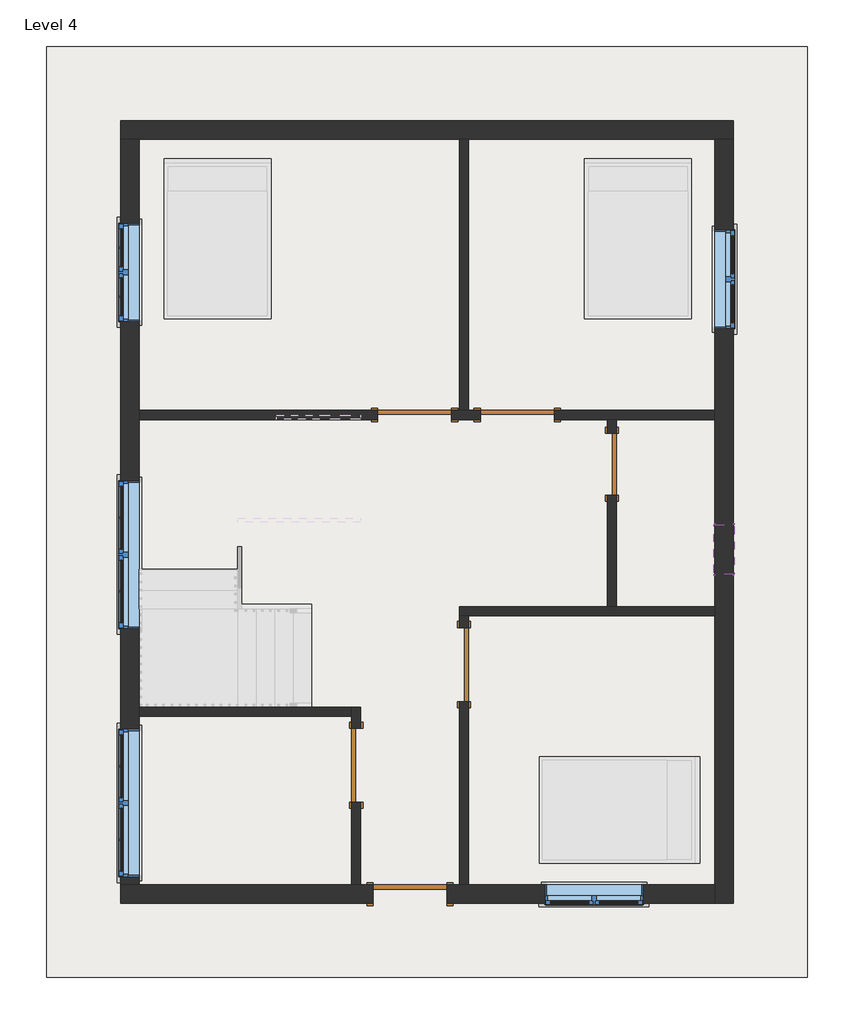
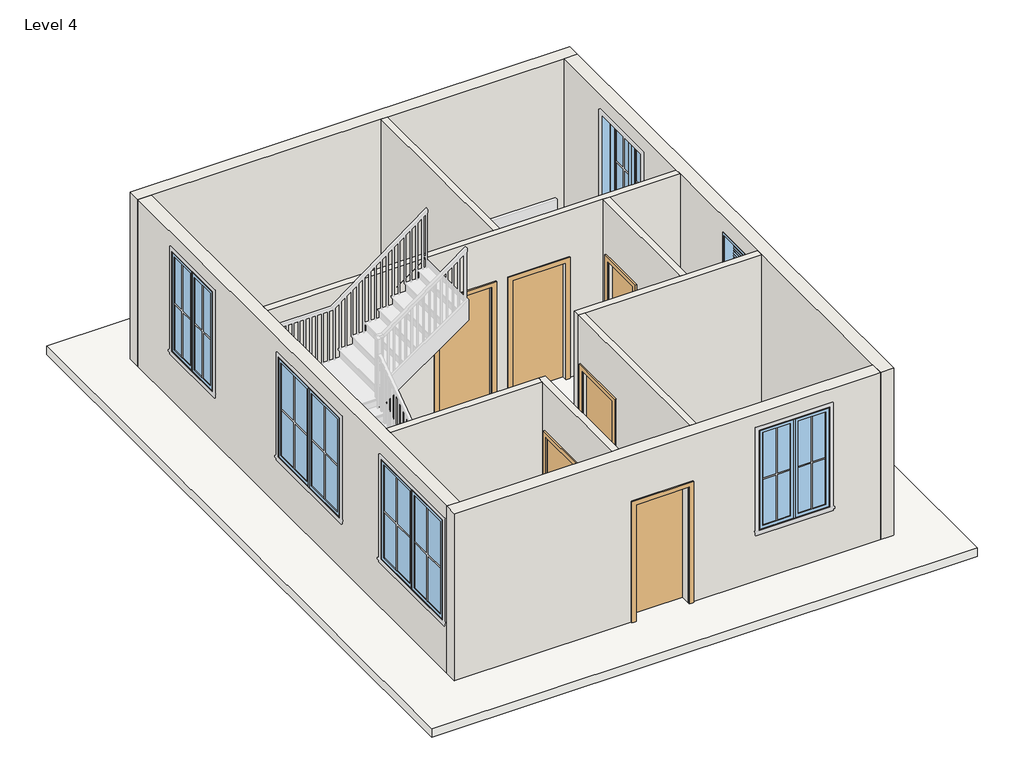
# One storey, part 1 of 3: 11 walls, 6 doors, 6 windows, 1 roof.
"""IFC4 building model written with IfcOpenShell, lengths in millimetres."""

from ifc_helpers import new_model, si_unit, frame, origin, place, context, project, spatial, polyline, outline, extrude, faceted_brep, transform, mapped, element, save
from components import door_f2b275c1, single_flush_door_3_e5f9f3c4, single_flush_door_3_305aa2a5, single_flush_door_3_a90ba1ad, window_casement_double_win_4_6ca1769e, window_casement_double_win_6_ce442eab, window_f2d8fef0

model = new_model("IFC4")

# Units and contexts
model_context = context("Model", 3, world=origin())
ifc_project = project(units=[si_unit("LENGTHUNIT", "METRE", prefix="MILLI")], contexts=[model_context])

# Site, building, storey
site = spatial("IfcSite", under=ifc_project)
building = spatial("IfcBuilding", under=site)
storey = spatial("IfcBuildingStorey", under=building, Name="Level 4", Elevation=9448.8)

# Doors
placement = place(None, origin())
door_shape = door_f2b275c1(model_context)
element("IfcDoor", 1, ObjectType="Single-Flush : 2'6\"", at=placement, inside=storey, context=model_context, shape_type="MappedRepresentation", body=[
    mapped(door_shape, transform((1031.6394609, 262.5126239, 9448.8), x_axis=(0.0, 1.0, 0.0), y_axis=(-1.0, 0.0, 0.0), z_axis=(0.0, 0.0, 1.0))),
])
single_flush_door_3_shape = single_flush_door_3_e5f9f3c4(model_context)
element("IfcDoor", 2, ObjectType="Single-Flush : door 3'", at=placement, inside=storey, context=model_context, shape_type="MappedRepresentation", body=[
    mapped(single_flush_door_3_shape, transform((-1406.7605391, 872.1126239, 9448.8), x_axis=(1.0, 0.0, 0.0), y_axis=(0.0, 1.0, 0.0), z_axis=(0.0, 0.0, 1.0))),
])
element("IfcDoor", 3, ObjectType="Single-Flush : door 3'", at=placement, inside=storey, context=model_context, shape_type="MappedRepresentation", body=[
    mapped(single_flush_door_3_shape, transform((-2130.6605391, -3458.5873761, 9448.8), x_axis=(0.0, 1.0, 0.0), y_axis=(-1.0, 0.0, 0.0), z_axis=(0.0, 0.0, 1.0))),
])
single_flush_door_3_2_shape = single_flush_door_3_305aa2a5(model_context)
element("IfcDoor", 4, ObjectType="Single-Flush : door 3'", at=placement, inside=storey, context=model_context, shape_type="MappedRepresentation", body=[
    mapped(single_flush_door_3_2_shape, transform((-136.7605391, 872.1126239, 9448.8), x_axis=(-1.0, 0.0, 0.0), y_axis=(0.0, -1.0, 0.0), z_axis=(0.0, 0.0, 1.0))),
])
element("IfcDoor", 5, ObjectType="Single-Flush : door 3'", at=placement, inside=storey, context=model_context, shape_type="MappedRepresentation", body=[
    mapped(single_flush_door_3_2_shape, transform((-797.1605391, -2213.9873761, 9448.8), x_axis=(0.0, 1.0, 0.0), y_axis=(-1.0, 0.0, 0.0), z_axis=(0.0, 0.0, 1.0))),
])
single_flush_door_3_3_shape = single_flush_door_3_a90ba1ad(model_context)
element("IfcDoor", 6, ObjectType="Single-Flush : door 3'", at=placement, inside=storey, context=model_context, shape_type="MappedRepresentation", body=[
    mapped(single_flush_door_3_3_shape, transform((-1463.9105391, -5052.4373761, 9448.8), x_axis=(-1.0, 0.0, 0.0), y_axis=(0.0, -1.0, 0.0), z_axis=(0.0, 0.0, 1.0))),
])

# Roof
element("IfcRoof", 7, ObjectType="Generic - 12\"", at=placement, inside=storey, context=model_context, shape_type="SweptSolid", body=[
    extrude(outline(polyline([(-5959.7105391, 5425.0626239), (3450.9894609, 5425.0626239), (3450.9894609, -6081.1373761), (-5959.7105391, -6081.1373761), (-5959.7105391, 5425.0626239)])), frame((0.0, 0.0, 9296.4), z_axis=(0.0, 0.0, 1.0), x_axis=(1.0, 0.0, 0.0)), (0.0, 0.0, 1.0), 152.4),
])

# Walls
element("IfcWall", 8, ObjectType="WALL 4.5\"", at=placement, inside=storey, context=model_context, shape_type="SweptSolid", body=[
    extrude(outline(polyline([(-854.3105391, 929.2626239), (-854.3105391, 4282.0626239), (-740.0105391, 4282.0626239), (-740.0105391, 929.2626239), (-854.3105391, 929.2626239)])), frame((0.0, 0.0, 9448.8), z_axis=(0.0, 0.0, 1.0), x_axis=(1.0, 0.0, 0.0)), (0.0, 0.0, 1.0), 3048.0),
])
element("IfcWall", 9, ObjectType="WALL 4.5\"", at=placement, inside=storey, context=model_context, shape_type="Brep", body=[
    faceted_brep([(-949.5605391, 814.9626239, 9448.8), (-593.9605391, 814.9626239, 9448.8), (-593.9605391, 814.9626239, 11582.4), (320.4394609, 814.9626239, 11582.4), (320.4394609, 814.9626239, 9448.8), (974.4894609, 814.9626239, 9448.8), (1088.7894609, 814.9626239, 9448.8), (2307.9894609, 814.9626239, 9448.8), (2307.9894609, 814.9626239, 12496.8), (1088.7894609, 814.9626239, 12496.8), (974.4894609, 814.9626239, 12496.8), (-4816.7105391, 814.9626239, 12496.8), (-4816.7105391, 814.9626239, 9448.8), (-1863.9605391, 814.9626239, 9448.8), (-1863.9605391, 814.9626239, 11582.4), (-949.5605391, 814.9626239, 11582.4), (-593.9605391, 929.2626239, 11582.4), (-593.9605391, 929.2626239, 9448.8), (-740.0105391, 929.2626239, 9448.8), (-854.3105391, 929.2626239, 9448.8), (-949.5605391, 929.2626239, 9448.8), (-949.5605391, 929.2626239, 11582.4), (-1863.9605391, 929.2626239, 11582.4), (-1863.9605391, 929.2626239, 9448.8), (-4816.7105391, 929.2626239, 9448.8), (-4816.7105391, 929.2626239, 12496.8), (-854.3105391, 929.2626239, 12496.8), (-740.0105391, 929.2626239, 12496.8), (2307.9894609, 929.2626239, 12496.8), (2307.9894609, 929.2626239, 9448.8), (320.4394609, 929.2626239, 9448.8), (320.4394609, 929.2626239, 11582.4)], [[[0, 1, 2, 3, 4, 5, 6, 7, 8, 9, 10, 11, 12, 13, 14, 15]], [[16, 17, 18, 19, 20, 21, 22, 23, 24, 25, 26, 27, 28, 29, 30, 31]], [[13, 12, 24, 23]], [[30, 29, 7, 6, 5, 4]], [[20, 19, 18, 17, 1, 0]], [[8, 7, 29, 28]], [[12, 11, 25, 24]], [[21, 20, 0, 15]], [[22, 21, 15, 14]], [[23, 22, 14, 13]], [[2, 1, 17, 16]], [[3, 2, 16, 31]], [[4, 3, 31, 30]], [[11, 10, 9, 8, 28, 27, 26, 25]]]),
])
element("IfcWall", 10, ObjectType="WALL 4.5\"", at=placement, inside=storey, context=model_context, shape_type="SweptSolid", body=[
    extrude(outline(polyline([(814.9626239, 9448.8), (643.5126239, 9448.8), (643.5126239, 11480.8), (-118.4873761, 11480.8), (-118.4873761, 9448.8), (-1496.4373761, 9448.8), (-1496.4373761, 12496.8), (814.9626239, 12496.8), (814.9626239, 9448.8)])), frame((974.4894609, 0.0, 0.0), z_axis=(1.0, 0.0, 0.0), x_axis=(0.0, 1.0, 0.0)), (0.0, 0.0, 1.0), 114.3),
])
element("IfcWall", 11, ObjectType="WALL 4.5\"", at=placement, inside=storey, context=model_context, shape_type="Brep", body=[
    faceted_brep([(2307.9894609, -1496.4373761, 9448.8), (1088.7894609, -1496.4373761, 9448.8), (974.4894609, -1496.4373761, 9448.8), (-854.3105391, -1496.4373761, 9448.8), (-854.3105391, -1496.4373761, 12496.8), (974.4894609, -1496.4373761, 12496.8), (1088.7894609, -1496.4373761, 12496.8), (2307.9894609, -1496.4373761, 12496.8), (2307.9894609, -1610.7373761, 9448.8), (2307.9894609, -1610.7373761, 12496.8), (-740.0105391, -1610.7373761, 12496.8), (-854.3105391, -1610.7373761, 12496.8), (-854.3105391, -1610.7373761, 9448.8), (-740.0105391, -1610.7373761, 9448.8)], [[[0, 1, 2, 3, 4, 5, 6, 7]], [[8, 9, 10, 11, 12, 13]], [[3, 2, 1, 0, 8, 13, 12]], [[0, 7, 9, 8]], [[4, 3, 12, 11]], [[7, 6, 5, 4, 11, 10, 9]]]),
])
element("IfcWall", 12, ObjectType="WALL 4.5\"", at=placement, inside=storey, context=model_context, shape_type="SweptSolid", body=[
    extrude(outline(polyline([(-1610.7373761, 9448.8), (-1756.7873761, 9448.8), (-1756.7873761, 11582.4), (-2671.1873761, 11582.4), (-2671.1873761, 9448.8), (-4938.1373761, 9448.8), (-4938.1373761, 12496.8), (-1610.7373761, 12496.8), (-1610.7373761, 9448.8)])), frame((-854.3105391, 0.0, 0.0), z_axis=(1.0, 0.0, 0.0), x_axis=(0.0, 1.0, 0.0)), (0.0, 0.0, 1.0), 114.3),
])
element("IfcWall", 13, ObjectType="WALL 4.5\"", at=placement, inside=storey, context=model_context, shape_type="Brep", body=[
    faceted_brep([(-2073.5105391, -3001.3873761, 11582.4), (-2073.5105391, -3001.3873761, 9448.8), (-2073.5105391, -2741.0373761, 9448.8), (-2073.5105391, -2741.0373761, 12496.8), (-2073.5105391, -4938.1373761, 12496.8), (-2073.5105391, -4938.1373761, 9448.8), (-2073.5105391, -3915.7873761, 9448.8), (-2073.5105391, -3915.7873761, 11582.4), (-2187.8105391, -2741.0373761, 9448.8), (-2187.8105391, -2855.3373761, 9448.8), (-2187.8105391, -3001.3873761, 9448.8), (-2187.8105391, -3001.3873761, 11582.4), (-2187.8105391, -3915.7873761, 11582.4), (-2187.8105391, -3915.7873761, 9448.8), (-2187.8105391, -4938.1373761, 9448.8), (-2187.8105391, -4938.1373761, 12496.8), (-2187.8105391, -2855.3373761, 12496.8), (-2187.8105391, -2741.0373761, 12496.8)], [[[0, 1, 2, 3, 4, 5, 6, 7]], [[8, 9, 10, 11, 12, 13, 14, 15, 16, 17]], [[6, 5, 14, 13]], [[2, 1, 10, 9, 8]], [[5, 4, 15, 14]], [[3, 2, 8, 17]], [[11, 10, 1, 0]], [[12, 11, 0, 7]], [[13, 12, 7, 6]], [[4, 3, 17, 16, 15]]]),
])
element("IfcWall", 14, ObjectType="WALL 4.5\"", at=placement, inside=storey, context=model_context, shape_type="SweptSolid", body=[
    extrude(outline(polyline([(-4816.7105391, -2741.0373761), (-2187.8105391, -2741.0373761), (-2187.8105391, -2855.3373761), (-4816.7105391, -2855.3373761), (-4816.7105391, -2741.0373761)])), frame((0.0, 0.0, 9448.8), z_axis=(0.0, 0.0, 1.0), x_axis=(1.0, 0.0, 0.0)), (0.0, 0.0, 1.0), 3048.0),
])
element("IfcWall", 15, ObjectType="WALL 9\"", at=placement, inside=storey, context=model_context, shape_type="Brep", body=[
    faceted_brep([(-5045.3105391, 4282.0626239, 9448.8), (-4816.7105391, 4282.0626239, 9448.8), (-854.3105391, 4282.0626239, 9448.8), (-740.0105391, 4282.0626239, 9448.8), (2307.9894609, 4282.0626239, 9448.8), (2536.5894609, 4282.0626239, 9448.8), (2536.5894609, 4282.0626239, 12496.8), (2307.9894609, 4282.0626239, 12496.8), (-740.0105391, 4282.0626239, 12496.8), (-854.3105391, 4282.0626239, 12496.8), (-4816.7105391, 4282.0626239, 12496.8), (-5045.3105391, 4282.0626239, 12496.8), (-5045.3105391, 4510.6626239, 9448.8), (-5045.3105391, 4510.6626239, 12496.8), (2536.5894609, 4510.6626239, 12496.8), (2536.5894609, 4510.6626239, 9448.8)], [[[0, 1, 2, 3, 4, 5, 6, 7, 8, 9, 10, 11]], [[12, 13, 14, 15]], [[5, 4, 3, 2, 1, 0, 12, 15]], [[6, 5, 15, 14]], [[0, 11, 13, 12]], [[11, 10, 9, 8, 7, 6, 14, 13]]]),
])
element("IfcWall", 16, ObjectType="WALL 9\"", at=placement, inside=storey, context=model_context, shape_type="Brep", body=[
    faceted_brep([(2307.9894609, 4282.0626239, 9448.8), (2307.9894609, 929.2626239, 9448.8), (2307.9894609, 814.9626239, 9448.8), (2307.9894609, -1496.4373761, 9448.8), (2307.9894609, -1610.7373761, 9448.8), (2307.9894609, -4938.1373761, 9448.8), (2307.9894609, -5166.7373761, 9448.8), (2307.9894609, -5166.7373761, 12496.8), (2307.9894609, -4938.1373761, 12496.8), (2307.9894609, -1610.7373761, 12496.8), (2307.9894609, -1496.4373761, 12496.8), (2307.9894609, 814.9626239, 12496.8), (2307.9894609, 929.2626239, 12496.8), (2307.9894609, 4282.0626239, 12496.8), (2307.9894609, 1938.9126239, 12192.0), (2307.9894609, 1938.9126239, 10363.2), (2307.9894609, 3158.1126239, 10363.2), (2307.9894609, 3158.1126239, 12192.0), (2307.9894609, -486.7873761, 12192.0), (2307.9894609, -1096.3873761, 12192.0), (2307.9894609, -1096.3873761, 11582.4), (2307.9894609, -486.7873761, 11582.4), (2536.5894609, 4282.0626239, 9448.8), (2536.5894609, 4282.0626239, 12496.8), (2536.5894609, -5166.7373761, 12496.8), (2536.5894609, -5166.7373761, 9448.8), (2536.5894609, 1938.9126239, 12192.0), (2536.5894609, 3158.1126239, 12192.0), (2536.5894609, 3158.1126239, 10363.2), (2536.5894609, 1938.9126239, 10363.2), (2536.5894609, -486.7873761, 12192.0), (2536.5894609, -486.7873761, 11582.4), (2536.5894609, -1096.3873761, 11582.4), (2536.5894609, -1096.3873761, 12192.0)], [[[0, 1, 2, 3, 4, 5, 6, 7, 8, 9, 10, 11, 12, 13], [14, 15, 16, 17], [18, 19, 20, 21]], [[22, 23, 24, 25], [26, 27, 28, 29], [30, 31, 32, 33]], [[6, 5, 4, 3, 2, 1, 0, 22, 25]], [[0, 13, 23, 22]], [[7, 6, 25, 24]], [[15, 14, 26, 29]], [[16, 15, 29, 28]], [[17, 16, 28, 27]], [[14, 17, 27, 26]], [[31, 30, 18, 21]], [[32, 31, 21, 20]], [[33, 32, 20, 19]], [[30, 33, 19, 18]], [[13, 12, 11, 10, 9, 8, 7, 24, 23]]]),
])
element("IfcWall", 17, ObjectType="WALL 9\"", at=placement, inside=storey, context=model_context, shape_type="Brep", body=[
    faceted_brep([(-1921.1105391, -4938.1373761, 11582.4), (-1921.1105391, -4938.1373761, 9448.8), (-2073.5105391, -4938.1373761, 9448.8), (-2187.8105391, -4938.1373761, 9448.8), (-4816.7105391, -4938.1373761, 9448.8), (-5045.3105391, -4938.1373761, 9448.8), (-5045.3105391, -4938.1373761, 12496.8), (-4816.7105391, -4938.1373761, 12496.8), (-2187.8105391, -4938.1373761, 12496.8), (-2073.5105391, -4938.1373761, 12496.8), (-854.3105391, -4938.1373761, 12496.8), (-740.0105391, -4938.1373761, 12496.8), (2307.9894609, -4938.1373761, 12496.8), (2307.9894609, -4938.1373761, 9448.8), (-740.0105391, -4938.1373761, 9448.8), (-854.3105391, -4938.1373761, 9448.8), (-1006.7105391, -4938.1373761, 9448.8), (-1006.7105391, -4938.1373761, 11582.4), (202.9644609, -4938.1373761, 12192.0), (202.9644609, -4938.1373761, 10363.2), (1422.1644609, -4938.1373761, 10363.2), (1422.1644609, -4938.1373761, 12192.0), (-5045.3105391, -5166.7373761, 9448.8), (-1921.1105391, -5166.7373761, 9448.8), (-1921.1105391, -5166.7373761, 11582.4), (-1006.7105391, -5166.7373761, 11582.4), (-1006.7105391, -5166.7373761, 9448.8), (2307.9894609, -5166.7373761, 9448.8), (2307.9894609, -5166.7373761, 12496.8), (-5045.3105391, -5166.7373761, 12496.8), (202.9644609, -5166.7373761, 12192.0), (1422.1644609, -5166.7373761, 12192.0), (1422.1644609, -5166.7373761, 10363.2), (202.9644609, -5166.7373761, 10363.2)], [[[0, 1, 2, 3, 4, 5, 6, 7, 8, 9, 10, 11, 12, 13, 14, 15, 16, 17], [18, 19, 20, 21]], [[22, 23, 24, 25, 26, 27, 28, 29], [30, 31, 32, 33]], [[5, 4, 3, 2, 1, 23, 22]], [[16, 15, 14, 13, 27, 26]], [[13, 12, 28, 27]], [[6, 5, 22, 29]], [[19, 18, 30, 33]], [[20, 19, 33, 32]], [[21, 20, 32, 31]], [[18, 21, 31, 30]], [[24, 23, 1, 0]], [[25, 24, 0, 17]], [[26, 25, 17, 16]], [[12, 11, 10, 9, 8, 7, 6, 29, 28]]]),
])
element("IfcWall", 18, ObjectType="WALL 9\"", at=placement, inside=storey, context=model_context, shape_type="Brep", body=[
    faceted_brep([(-4816.7105391, -4938.1373761, 9448.8), (-4816.7105391, -2855.3373761, 9448.8), (-4816.7105391, -2741.0373761, 9448.8), (-4816.7105391, 814.9626239, 9448.8), (-4816.7105391, 929.2626239, 9448.8), (-4816.7105391, 4282.0626239, 9448.8), (-4816.7105391, 4282.0626239, 12496.8), (-4816.7105391, 929.2626239, 12496.8), (-4816.7105391, 814.9626239, 12496.8), (-4816.7105391, -2741.0373761, 12496.8), (-4816.7105391, -2855.3373761, 12496.8), (-4816.7105391, -4938.1373761, 12496.8), (-4816.7105391, -3010.9123761, 12192.0), (-4816.7105391, -3010.9123761, 10363.2), (-4816.7105391, -4839.7123761, 10363.2), (-4816.7105391, -4839.7123761, 12192.0), (-4816.7105391, 59.3126239, 12192.0), (-4816.7105391, 59.3126239, 10363.2), (-4816.7105391, -1769.4873761, 10363.2), (-4816.7105391, -1769.4873761, 12192.0), (-4816.7105391, 3243.8376239, 12192.0), (-4816.7105391, 3243.8376239, 10363.2), (-4816.7105391, 2024.6376239, 10363.2), (-4816.7105391, 2024.6376239, 12192.0), (-5045.3105391, -4938.1373761, 9448.8), (-5045.3105391, -4938.1373761, 12496.8), (-5045.3105391, 4282.0626239, 12496.8), (-5045.3105391, 4282.0626239, 9448.8), (-5045.3105391, -3010.9123761, 12192.0), (-5045.3105391, -4839.7123761, 12192.0), (-5045.3105391, -4839.7123761, 10363.2), (-5045.3105391, -3010.9123761, 10363.2), (-5045.3105391, 59.3126239, 12192.0), (-5045.3105391, -1769.4873761, 12192.0), (-5045.3105391, -1769.4873761, 10363.2), (-5045.3105391, 59.3126239, 10363.2), (-5045.3105391, 3243.8376239, 12192.0), (-5045.3105391, 2024.6376239, 12192.0), (-5045.3105391, 2024.6376239, 10363.2), (-5045.3105391, 3243.8376239, 10363.2)], [[[0, 1, 2, 3, 4, 5, 6, 7, 8, 9, 10, 11], [12, 13, 14, 15], [16, 17, 18, 19], [20, 21, 22, 23]], [[24, 25, 26, 27], [28, 29, 30, 31], [32, 33, 34, 35], [36, 37, 38, 39]], [[5, 4, 3, 2, 1, 0, 24, 27]], [[6, 5, 27, 26]], [[0, 11, 25, 24]], [[13, 12, 28, 31]], [[14, 13, 31, 30]], [[15, 14, 30, 29]], [[12, 15, 29, 28]], [[17, 16, 32, 35]], [[18, 17, 35, 34]], [[19, 18, 34, 33]], [[16, 19, 33, 32]], [[21, 20, 36, 39]], [[22, 21, 39, 38]], [[23, 22, 38, 37]], [[20, 23, 37, 36]], [[11, 10, 9, 8, 7, 6, 26, 25]]]),
])

# Windows
window_casement_double_win_4_shape = window_casement_double_win_4_6ca1769e(model_context)
element("IfcWindow", 19, ObjectType="Window-Casement-Double : win 4'", at=placement, inside=storey, context=model_context, shape_type="MappedRepresentation", body=[
    mapped(window_casement_double_win_4_shape, transform((812.5644609, -5052.4373761, 9448.8), x_axis=(-1.0, 0.0, 0.0), y_axis=(0.0, -1.0, 0.0), z_axis=(0.0, 0.0, 1.0))),
])
element("IfcWindow", 20, ObjectType="Window-Casement-Double : win 4'", at=placement, inside=storey, context=model_context, shape_type="MappedRepresentation", body=[
    mapped(window_casement_double_win_4_shape, transform((2422.2894609, 2548.5126239, 9448.8), x_axis=(0.0, -1.0, 0.0), y_axis=(1.0, 0.0, 0.0), z_axis=(0.0, 0.0, 1.0))),
])
element("IfcWindow", 21, ObjectType="Window-Casement-Double : win 4'", at=placement, inside=storey, context=model_context, shape_type="MappedRepresentation", body=[
    mapped(window_casement_double_win_4_shape, transform((-4931.0105391, 2634.2376239, 9448.8), x_axis=(0.0, 1.0, 0.0), y_axis=(-1.0, 0.0, 0.0), z_axis=(0.0, 0.0, 1.0))),
])
window_casement_double_win_6_shape = window_casement_double_win_6_ce442eab(model_context)
element("IfcWindow", 22, ObjectType="Window-Casement-Double : win 6'", at=placement, inside=storey, context=model_context, shape_type="MappedRepresentation", body=[
    mapped(window_casement_double_win_6_shape, transform((-4931.0105391, -3925.3123761, 9448.8), x_axis=(0.0, 1.0, 0.0), y_axis=(-1.0, 0.0, 0.0), z_axis=(0.0, 0.0, 1.0))),
])
element("IfcWindow", 23, ObjectType="Window-Casement-Double : win 6'", at=placement, inside=storey, context=model_context, shape_type="MappedRepresentation", body=[
    mapped(window_casement_double_win_6_shape, transform((-4931.0105391, -855.0873761, 9448.8), x_axis=(0.0, 1.0, 0.0), y_axis=(-1.0, 0.0, 0.0), z_axis=(0.0, 0.0, 1.0))),
])
window_shape = window_f2d8fef0(model_context)
element("IfcWindow", 24, ObjectType="Window-Louvers : 24\" x 24\"", at=placement, inside=storey, context=model_context, shape_type="MappedRepresentation", body=[
    mapped(window_shape, transform((2428.6394609, -791.5873761, 10668.0), x_axis=(0.0, -1.0, 0.0), y_axis=(1.0, 0.0, 0.0), z_axis=(0.0, 0.0, 1.0))),
])

save(model, "model.ifc")

# Revit data of these elements
# Type "Single-Flush : 2'6\""
#   Type Mark = "9"
#   Construction Type Id = "MDOOR"
#   Assembly Code = "C1020"
#   Analytic Construction = "Metal"
#   Thickness = 0' - 2"
#   Heat Transfer Coefficient (U) = 0.651978 BTU/(h·ft²·°F)
#   Height = 6' - 8"
#   Trim Projection Ext = 0' - 1"
#   Trim Projection Int = 0' - 1"
#   Trim Width = 0' - 3"
#   Width = 2' - 6"
#   Define Thermal Properties by = 1
#   Door Material = Door - Panel
#   Frame Material = Door - Frame
#   Visual Light Transmittance = 0
#   Solar Heat Gain Coefficient = 0
#   Function = (empty or 0)
#   Wall Closure = (empty or 0)
# Type "Single-Flush : door 3'"
#   Type Mark = "8"
#   Construction Type Id = "MDOOR"
#   Assembly Code = "C1020"
#   Analytic Construction = "Metal"
#   Thickness = 0' - 2"
#   Heat Transfer Coefficient (U) = 0.651978 BTU/(h·ft²·°F)
#   Height = 7' - 0"
#   Trim Projection Ext = 0' - 1"
#   Trim Projection Int = 0' - 1"
#   Trim Width = 0' - 3"
#   Width = 3' - 0"
#   Define Thermal Properties by = 1
#   Door Material = Door - Panel
#   Frame Material = Door - Frame
#   Visual Light Transmittance = 0
#   Solar Heat Gain Coefficient = 0
#   Function = (empty or 0)
#   Wall Closure = (empty or 0)
# Type "Generic - 12\""
#   Assembly Code = "B1020"
#   Layers, outside or top first: 0' - 6" no material (function 1)
# Type "WALL 4.5\""
#   Assembly Code = "B2010"
#   Layers, outside or top first: 0' - 4 1/2" no material (function 1)
# Type "WALL 9\""
#   Assembly Code = "B2010"
#   Layers, outside or top first: 0' - 9" no material (function 1)
# Type "Window-Casement-Double : win 4'"
#   Type Mark = "19"
#   Fire Rating = "0.5h"
#   Assembly Code = "B2020100"
#   Analytic Construction = "Double glazing - domestic"
#   Frame Extension [instance default] = 0' - 0 1/4"
#   Window Inset [instance default] = 0' - 0"
#   Wall Thickness [instance default] = 0' - 6"
#   Interior Wall Closure [instance default] = 0' - 2 1/4"
#   Half Width = 2' - 0"
#   Visual Light Transmittance = 0.81
#   Thermal Resistance (R) = 1.8146 (h·ft²·°F)/BTU
#   Solar Heat Gain Coefficient = 0.76
#   Rough Width = 4' - 0 1/2"
#   Rough Height = 6' - 0 1/2"
#   Height = 6' - 0"
#   Heat Transfer Coefficient (U) = 0.5511 BTU/(h·ft²·°F)
#   Exterior Wall Closure [instance default] = 0' - 1 1/4"
#   Extension Jamb [instance default] = 0' - 2 1/4"
#   Default Sill Height = 3' - 0"
#   Width = 4' - 0"
#   Muntin Visibility = yes
#   Interior Trim Visibility [instance default] = yes
#   Exterior Trim Visibility [instance default] = yes
#   Extension Jamb Visibility [instance default] = yes
#   Interior Trim Material = Wood - Stained
#   Muntin Pattern = Muntin Pattern_2x2 : Muntin Pattern_2x2
#   Interior Trim = Trim-Window-Interior-Flat : Picture Frame
#   Interior Frame Material = Wood - Stained
#   Glass Panel Material = Glass
#   Exterior Trim Material = Clad - White
#   Exterior Trim = Trim-Window-Exterior-Flat : with Sill
#   Exterior Frame Material = Clad - White
#   Wall Closure = (empty or 0)
# Type "Window-Casement-Double : win 6'"
#   Type Mark = "18"
#   Fire Rating = "0.5h"
#   Assembly Code = "B2020100"
#   Analytic Construction = "Double glazing - domestic"
#   Frame Extension [instance default] = 0' - 0 1/4"
#   Window Inset [instance default] = 0' - 0"
#   Wall Thickness [instance default] = 0' - 6"
#   Interior Wall Closure [instance default] = 0' - 2 1/4"
#   Half Width = 3' - 0"
#   Visual Light Transmittance = 0.81
#   Thermal Resistance (R) = 1.8146 (h·ft²·°F)/BTU
#   Solar Heat Gain Coefficient = 0.76
#   Rough Width = 6' - 0 1/2"
#   Rough Height = 6' - 0 1/2"
#   Height = 6' - 0"
#   Heat Transfer Coefficient (U) = 0.5511 BTU/(h·ft²·°F)
#   Exterior Wall Closure [instance default] = 0' - 1 1/4"
#   Extension Jamb [instance default] = 0' - 2 1/4"
#   Default Sill Height = 3' - 0"
#   Width = 6' - 0"
#   Muntin Visibility = yes
#   Interior Trim Visibility [instance default] = yes
#   Exterior Trim Visibility [instance default] = yes
#   Extension Jamb Visibility [instance default] = yes
#   Interior Trim Material = Wood - Stained
#   Muntin Pattern = Muntin Pattern_2x2 : Muntin Pattern_2x2
#   Interior Trim = Trim-Window-Interior-Flat : Picture Frame
#   Interior Frame Material = Wood - Stained
#   Glass Panel Material = Glass
#   Exterior Trim Material = Clad - White
#   Exterior Trim = Trim-Window-Exterior-Flat : with Sill
#   Exterior Frame Material = Clad - White
#   Wall Closure = (empty or 0)
# Type "Window-Louvers : 24\" x 24\""
#   Type Mark = "20"
#   Construction Type Id = "GSP4R"
#   Assembly Code = "B20"
#   Analytic Construction = "1/8 in Pilkington single glazing"
#   Visual Light Transmittance = 0.9
#   Thermal Resistance (R) = 1.53941 (h·ft²·°F)/BTU
#   Solar Heat Gain Coefficient = 0.78
#   Max Height = 1' - 11.74264"
#   Height = 2' - 0"
#   Heat Transfer Coefficient (U) = 0.6496 BTU/(h·ft²·°F)
#   Blade Width [instance default] = 1' - 10 1/2"
#   Blade Vertical Thickness = 0' - 0.35355"
#   Blade Thickness = 0' - 0 1/4"
#   Blade Spacing = 0' - 1 1/2"
#   Blade Height = 0' - 1.85355"
#   Blade Depth = 0' - 3"
#   Blade Angle = 45.00°
#   Default Sill Height = 3' - 0"
#   Trim Projection_Exterior = 0' - 0 1/2"
#   Trim Projection_Interior = 0' - 0 1/2"
#   Trim Width_Exterior = 0' - 1 1/2"
#   Trim Width_Interior = 0' - 1 1/2"
#   Width = 2' - 0"
#   Max Blade Count = 12
#   Define Thermal Properties by = 1
#   Blade Count = 12
#   Frame Material = Birch
#   Louver Material = Birch
#   Trim Exterior Material = Birch
#   Trim Interior Material = Birch
#   Wall Closure = (empty or 0)
# Element 1 (IfcDoor, "Single-Flush : 2'6\"")
#   Phase Created = New Construction
#   Materials on its faces: "Door - Frame", "Door - Panel"
# Elements 2, 3, 4, 5, 6 (IfcDoor, "Single-Flush : door 3'")
#   Phase Created = New Construction
#   Materials on its faces: "Door - Frame", "Door - Panel"
# Element 7 (IfcRoof, "Generic - 12\"")
#   built-in parameter 1001705 = 31 (stored number, unit not read)
#   built-in parameter 1001701 = -0.5 (stored number, unit not read)
#   built-in parameter 1001710 = 33615
#   Phase Created = New Construction
#   Materials on its faces: "Wood Planks", "Wood - Stained"
# Elements 8, 9, 10, 11, 12, 13, 14 (IfcWall, "WALL 4.5\"")
#   Top Offset = 0' - 0"
#   Base Offset = 0' - 0"
#   Unconnected Height = 10' - 0"
#   wall height = 10' - 0"
#   Phase Created = New Construction
#   Base Constraint = Level 4
#   Materials on its faces: "Default Wall"
# Elements 15, 16, 17, 18 (IfcWall, "WALL 9\"")
#   Top Offset = 0' - 0"
#   Base Offset = 0' - 0"
#   Unconnected Height = 10' - 0"
#   wall height = 10' - 0"
#   Phase Created = New Construction
#   Base Constraint = Level 4
#   Materials on its faces: "Default Wall", "Door - Frame"
# Element 19 (IfcWindow, "Window-Casement-Double : win 4'")
#   Mark = "21"
#   Window Inset = 0' - 0"
#   Interior Wall Closure = 0' - 2 1/4"
#   Frame Extension = 0' - 0 1/4"
#   Exterior Wall Closure = 0' - 1 1/4"
#   Interior Trim Visibility = yes
#   Exterior Trim Visibility = yes
#   Phase Created = New Construction
#   Materials on its faces: "Wood - Stained", "Glass", "Clad - White"
# Element 20 (IfcWindow, "Window-Casement-Double : win 4'")
#   Mark = "22"
#   Window Inset = 0' - 0"
#   Interior Wall Closure = 0' - 2 1/4"
#   Frame Extension = 0' - 0 1/4"
#   Exterior Wall Closure = 0' - 1 1/4"
#   Interior Trim Visibility = yes
#   Exterior Trim Visibility = yes
#   Phase Created = New Construction
#   Materials on its faces: "Wood - Stained", "Glass", "Clad - White"
# Element 21 (IfcWindow, "Window-Casement-Double : win 4'")
#   Mark = "23"
#   Window Inset = 0' - 0"
#   Interior Wall Closure = 0' - 2 1/4"
#   Frame Extension = 0' - 0 1/4"
#   Exterior Wall Closure = 0' - 1 1/4"
#   Interior Trim Visibility = yes
#   Exterior Trim Visibility = yes
#   Phase Created = New Construction
#   Materials on its faces: "Wood - Stained", "Glass", "Clad - White"
# Element 22 (IfcWindow, "Window-Casement-Double : win 6'")
#   Mark = "19"
#   Window Inset = 0' - 0"
#   Interior Wall Closure = 0' - 2 1/4"
#   Frame Extension = 0' - 0 1/4"
#   Exterior Wall Closure = 0' - 1 1/4"
#   Interior Trim Visibility = yes
#   Exterior Trim Visibility = yes
#   Phase Created = New Construction
#   Materials on its faces: "Wood - Stained", "Glass", "Clad - White"
# Element 23 (IfcWindow, "Window-Casement-Double : win 6'")
#   Mark = "20"
#   Window Inset = 0' - 0"
#   Interior Wall Closure = 0' - 2 1/4"
#   Frame Extension = 0' - 0 1/4"
#   Exterior Wall Closure = 0' - 1 1/4"
#   Interior Trim Visibility = yes
#   Exterior Trim Visibility = yes
#   Phase Created = New Construction
#   Materials on its faces: "Wood - Stained", "Glass", "Clad - White"
# Element 24 (IfcWindow, "Window-Louvers : 24\" x 24\"")
#   Mark = "24"
#   Blade Width = 1' - 10 1/2"
#   Phase Created = New Construction
#   Materials on its faces: "Birch"
# Materials
#   "Door - Panel": class "Wood", colour RGB 210 159 95, transparency 0, Cost = 0
#   "Door - Frame": colour RGB 118 70 51, transparency 0, Cost = 0
#   "Wood - Stained": class "Wood", colour RGB 224 178 126, transparency 0, Cost = 0
#   "Glass": class "Glass", colour RGB 0 128 192, transparency 0.75, Description = "Soda Lime Glass", Cost = 0
#   "Clad - White": class "Wood", colour RGB 242 242 238, transparency 0, Cost = 0
#   "Birch": class "Wood", colour RGB 224 178 126, transparency 0, Description = "Betula Alleghaniensis", Cost = 0
#   "Wood Planks": class "Wood", colour RGB 193 160 115, transparency 0, Description = "Physical material.", Cost = 0
#   "Default Wall": colour RGB 128 128 128, transparency 0, Cost = 0
